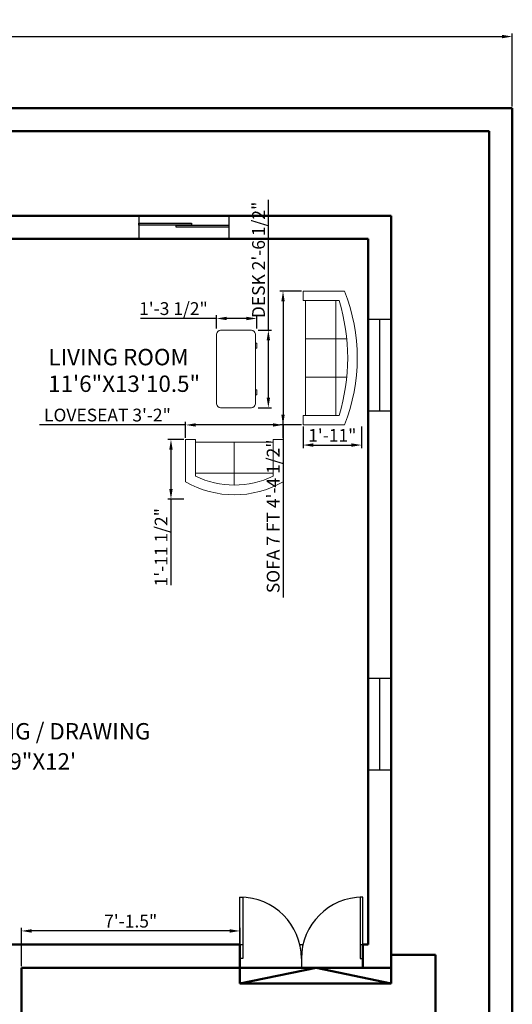
# Model space of a CAD drawing. Units: inches. Extents: x 116541 to 117938, y 135634 to 136328.
# Tile 4 of 9: x 116838 to 117030, y 135936 to 136321. Entities that reach past the tile are written whole.
import ezdxf

# ---------------------------------------------------------------- set-up
doc = ezdxf.new("R2010")
doc.units = ezdxf.units.IN
for name, color, linetype, lineweight in [('A-ANNO-DIMS', 2, 'Continuous', 18), ('A-AREA-IDEN', 3, 'Continuous', 25), ('A-DOOR', 4, 'Continuous', 25), ('A-FURN', 8, 'Continuous', 18), ('A-GLAZ', 1, 'Continuous', 25), ('A-WALL', 7, 'Continuous', 50)]:
    doc.layers.add(name, color=color, linetype=linetype, lineweight=lineweight)
doc.styles.get("Standard").update_dxf_attribs({"font": 'arial.ttf'})
doc.dimstyles.new('ISO-25', dxfattribs={"dimtxt": 5, "dimasz": 4, "dimexe": 1.25, "dimexo": 0.625, "dimtad": 1, "dimdec": 3, "dimlunit": 3, "dimtxsty": 'Standard', "dimcen": 2.5, "dimadec": 0, "dimazin": 0, "dimtfac": 1, "dimtdec": 3, "dimtmove": 0, "dimatfit": 3, "dimfxl": 1, "dimarcsym": 0})

# ---------------------------------------------------------------- blocks, each defined once
blk = doc.blocks.new('*U2')
for p, q in [((0, 0), (0, -6)), ((40, 0), (40, -6))]:
    blk.add_line(p, q)
blk.add_lwpolyline([(0, 0), (0, 40), (1.75, 40), (1.75, 0)], close=True)
blk.add_arc((0, 0), 40, 0, 90)
blk = doc.blocks.new('*U3')
for p, q in [((0, 0), (0, -6)), ((-40, 0), (-40, -6))]:
    blk.add_line(p, q)
blk.add_lwpolyline([(0, 0), (0, 40), (-1.75, 40), (-1.75, 0)], close=True)
blk.add_arc((0, 0), 40, 90, 180)
blk = doc.blocks.new('Sofa - Roundback 7 ft.')
for p, q in [((-36.000027, -34), (-36.000027, -11.4696)), ((-12.00002, -32.4421), (-12.00003, -6.5971)), ((11.99997, -32.4421), (11.99998, -6.5971)), ((35.99998, -34), (35.99998, -11.4696)), ((-35.999844, -13.3819), (35.9998, -13.3819)), ((-36.000027, -32.4421), (35.99998, -32.4421))]:
    blk.add_line(p, q)
for points in [[(-36.000027, -34), (-42.000027, -34), (-42.000027, -8)], [(41.99998, -8), (41.99998, -34), (35.99998, -34)]]:
    blk.add_lwpolyline(points)
for centre, radius, start, end in [((0, -114.25), 114.25, 68.43141, 111.5686), ((-0.00001, -127.1968), 121.1968, 72.72033, 107.2797)]:
    blk.add_arc(centre, radius, start, end)
blk = doc.blocks.new('Sofa - Roundback Loveseat 5 ft.')
for p, q in [((0, -32.44198), (0, -5.99998)), ((-24, -33.99998), (-24, -11.46958)), ((24.00004, -33.99998), (24.00004, -11.46958)), ((-23.9998, -13.38178), (23.99986, -13.38178)), ((-24, -32.44198), (24.00004, -32.44198))]:
    blk.add_line(p, q)
for points in [[(-24, -33.99998), (-30, -33.99998), (-30, -7.99998)], [(30.00004, -7.99998), (30.00004, -33.99998), (24.00004, -33.99998)]]:
    blk.add_lwpolyline(points)
for centre, radius, start, end in [((0, -60.24998), 60.24998, 60.13715, 119.8628), ((0, -61.38438), 55.38444, 64.32083, 115.6792)]:
    blk.add_arc(centre, radius, start, end)
blk = doc.blocks.new('Desk - 30 x 60 in.')
for p, q in [((-26.999995, 0), (26.999995, 0)), ((-29.999995, -27), (-29.999995, -3)), ((29.999995, -3), (29.999995, -27)), ((26.999995, -30), (-26.999995, -30)), ((-20.000005, -30), (-20.000005, -31)), ((-16.000005, -31), (-16.000005, -30)), ((15.999995, -31), (15.999995, -30)), ((19.999995, -30), (19.999995, -31)), ((-20.000005, -31), (-16.000005, -31)), ((19.999995, -31), (15.999995, -31))]:
    blk.add_line(p, q)
for centre, start, end in [((-26.499995, -3.5), 98.1301, 171.8699), ((26.499995, -3.5), 8.130102, 81.8699), ((-26.499995, -26.5), 188.1301, 261.8699), ((26.499995, -26.5), 278.1301, 351.8699)]:
    blk.add_arc(centre, 3.535534, start, end)
blk = doc.blocks.new('*D27')
at = {"layer": 'A-ANNO-DIMS', "color": 0, "lineweight": -2, "transparency": 16777216}
for p, q in [((116583.18, 136287.13), (116583.18, 136315.79)), ((116587.18, 136314.54), (117026.18, 136314.54)), ((117030.18, 136287.13), (117030.18, 136315.79))]:
    blk.add_line(p, q, dxfattribs=at)
at = {"layer": 'A-ANNO-DIMS', "color": 0, "transparency": 16777216}
for points in [[(116587.18, 136315.21), (116587.18, 136313.88), (116583.18, 136314.54)], [(117026.18, 136315.21), (117026.18, 136313.88), (117030.18, 136314.54)]]:
    blk.add_solid(points, dxfattribs=at)
at = {"layer": 'Defpoints', "color": 0, "transparency": 16777216}
for p in [(117030.18, 136314.54), (116583.18, 136286.5), (117030.18, 136286.5)]:
    blk.add_point(p, dxfattribs=at)
at = {"layer": 'A-ANNO-DIMS', "color": 0, "transparency": 16777216, "insert": (116806.68, 136317.72), "char_height": 5, "attachment_point": 5}
blk.add_mtext('37\'-3"', dxfattribs=at)
blk = doc.blocks.new('*D28')
at = {"layer": 'A-ANNO-DIMS', "color": 0, "lineweight": -2, "transparency": 16777216}
for p, q in [((116838.18, 135951.13), (116838.18, 135966.12)), ((116923.68, 135951.13), (116923.68, 135966.12)), ((116919.68, 135964.87), (116842.18, 135964.87))]:
    blk.add_line(p, q, dxfattribs=at)
at = {"layer": 'A-ANNO-DIMS', "color": 0, "transparency": 16777216}
for points in [[(116842.18, 135965.54), (116842.18, 135964.2), (116838.18, 135964.87)], [(116919.68, 135965.54), (116919.68, 135964.2), (116923.68, 135964.87)]]:
    blk.add_solid(points, dxfattribs=at)
at = {"layer": 'Defpoints', "color": 0, "transparency": 16777216}
for p in [(116838.18, 135964.87), (116838.18, 135950.5), (116923.68, 135950.5)]:
    blk.add_point(p, dxfattribs=at)
at = {"layer": 'A-ANNO-DIMS', "color": 0, "transparency": 16777216, "insert": (116880.93, 135968.05), "char_height": 5, "attachment_point": 5}
blk.add_mtext('7\'-1.5"', dxfattribs=at)
blk = doc.blocks.new('*D88')
at = {"layer": 'A-ANNO-DIMS', "color": 0, "lineweight": -2, "transparency": 16777216}
for p, q in [((116947.73, 136215.04), (116939.25, 136215.04)), ((116940.5, 136211.04), (116940.5, 136166.68)), ((116947.73, 136162.68), (116939.25, 136162.68)), ((116940.5, 136162.68), (116940.5, 136095.26))]:
    blk.add_line(p, q, dxfattribs=at)
at = {"layer": 'A-ANNO-DIMS', "color": 0, "transparency": 16777216}
for points in [[(116939.84, 136211.04), (116941.17, 136211.04), (116940.5, 136215.04)], [(116939.84, 136166.68), (116941.17, 136166.68), (116940.5, 136162.68)]]:
    blk.add_solid(points, dxfattribs=at)
at = {"layer": 'Defpoints', "color": 0, "transparency": 16777216}
for p in [(116948.36, 136215.04), (116940.5, 136162.68), (116948.36, 136162.68)]:
    blk.add_point(p, dxfattribs=at)
at = {"layer": 'A-ANNO-DIMS', "color": 0, "transparency": 16777216, "insert": (116937.29, 136126.97), "char_height": 5, "attachment_point": 5, "rotation": 90}
blk.add_mtext('SOFA 7 FT 4\'-4 1/2"', dxfattribs=at)
blk = doc.blocks.new('*D89')
at = {"layer": 'A-ANNO-DIMS', "color": 0, "lineweight": -2, "transparency": 16777216}
for p, q in [((116948.36, 136162.06), (116948.36, 136153.58)), ((116971.21, 136162.06), (116971.21, 136153.58)), ((116952.36, 136154.83), (116967.21, 136154.83))]:
    blk.add_line(p, q, dxfattribs=at)
at = {"layer": 'A-ANNO-DIMS', "color": 0, "transparency": 16777216}
for points in [[(116952.36, 136155.5), (116952.36, 136154.16), (116948.36, 136154.83)], [(116967.21, 136155.5), (116967.21, 136154.16), (116971.21, 136154.83)]]:
    blk.add_solid(points, dxfattribs=at)
at = {"layer": 'Defpoints', "color": 0, "transparency": 16777216}
for p in [(116948.36, 136162.68), (116971.21, 136162.68), (116971.21, 136154.83)]:
    blk.add_point(p, dxfattribs=at)
at = {"layer": 'A-ANNO-DIMS', "color": 0, "transparency": 16777216, "insert": (116959.78, 136157.97), "char_height": 5, "attachment_point": 5}
blk.add_mtext('1\'-11"', dxfattribs=at)
blk = doc.blocks.new('*D90')
at = {"layer": 'A-ANNO-DIMS', "color": 0, "lineweight": -2, "transparency": 16777216}
for p, q in [((116902.4, 136162.69), (116845.26, 136162.69)), ((116902.4, 136157.6), (116902.4, 136163.94)), ((116936.52, 136162.69), (116906.4, 136162.69)), ((116940.52, 136157.6), (116940.52, 136163.94))]:
    blk.add_line(p, q, dxfattribs=at)
at = {"layer": 'A-ANNO-DIMS', "color": 0, "transparency": 16777216}
for points in [[(116906.4, 136163.36), (116906.4, 136162.03), (116902.4, 136162.69)], [(116936.52, 136163.36), (116936.52, 136162.03), (116940.52, 136162.69)]]:
    blk.add_solid(points, dxfattribs=at)
at = {"layer": 'Defpoints', "color": 0, "transparency": 16777216}
for p in [(116902.4, 136162.69), (116902.4, 136156.97), (116940.52, 136156.97)]:
    blk.add_point(p, dxfattribs=at)
at = {"layer": 'A-ANNO-DIMS', "color": 0, "transparency": 16777216, "insert": (116871.83, 136165.91), "char_height": 5, "attachment_point": 5}
blk.add_mtext('LOVESEAT 3\'-2"', dxfattribs=at)
blk = doc.blocks.new('*D91')
at = {"layer": 'A-ANNO-DIMS', "color": 0, "lineweight": -2, "transparency": 16777216}
for p, q in [((116901.77, 136156.97), (116895.43, 136156.97)), ((116896.68, 136152.97), (116896.68, 136137.68)), ((116901.77, 136133.68), (116895.43, 136133.68)), ((116896.68, 136133.68), (116896.68, 136100.07))]:
    blk.add_line(p, q, dxfattribs=at)
at = {"layer": 'A-ANNO-DIMS', "color": 0, "transparency": 16777216}
for points in [[(116896.01, 136152.97), (116897.35, 136152.97), (116896.68, 136156.97)], [(116896.01, 136137.68), (116897.35, 136137.68), (116896.68, 136133.68)]]:
    blk.add_solid(points, dxfattribs=at)
at = {"layer": 'Defpoints', "color": 0, "transparency": 16777216}
for p in [(116902.4, 136156.97), (116896.68, 136133.68), (116902.4, 136133.68)]:
    blk.add_point(p, dxfattribs=at)
at = {"layer": 'A-ANNO-DIMS', "color": 0, "transparency": 16777216, "insert": (116893.47, 136114.88), "char_height": 5, "attachment_point": 5, "rotation": 90}
blk.add_mtext('1\'-11 1/2"', dxfattribs=at)
blk = doc.blocks.new('*D92')
at = {"layer": 'A-ANNO-DIMS', "color": 0, "lineweight": -2, "transparency": 16777216}
for p, q in [((116934.77, 136199.76), (116934.77, 136250.66)), ((116930.84, 136199.76), (116936.02, 136199.76)), ((116934.77, 136173.37), (116934.77, 136195.76)), ((116930.84, 136169.37), (116936.02, 136169.37))]:
    blk.add_line(p, q, dxfattribs=at)
at = {"layer": 'A-ANNO-DIMS', "color": 0, "transparency": 16777216}
for points in [[(116934.1, 136195.76), (116935.44, 136195.76), (116934.77, 136199.76)], [(116934.1, 136173.37), (116935.44, 136173.37), (116934.77, 136169.37)]]:
    blk.add_solid(points, dxfattribs=at)
at = {"layer": 'Defpoints', "color": 0, "transparency": 16777216}
for p in [(116930.21, 136199.76), (116934.77, 136199.76), (116930.21, 136169.37)]:
    blk.add_point(p, dxfattribs=at)
at = {"layer": 'A-ANNO-DIMS', "color": 0, "transparency": 16777216, "insert": (116931.56, 136227.21), "char_height": 5, "attachment_point": 5, "rotation": 90}
blk.add_mtext('DESK 2\'-6 1/2"', dxfattribs=at)
blk = doc.blocks.new('*D93')
at = {"layer": 'A-ANNO-DIMS', "color": 0, "lineweight": -2, "transparency": 16777216}
for p, q in [((116914.51, 136200.38), (116914.51, 136205.57)), ((116930.21, 136200.38), (116930.21, 136205.57)), ((116914.51, 136204.32), (116884.79, 136204.32)), ((116926.21, 136204.32), (116918.51, 136204.32))]:
    blk.add_line(p, q, dxfattribs=at)
at = {"layer": 'A-ANNO-DIMS', "color": 0, "transparency": 16777216}
for points in [[(116918.51, 136204.98), (116918.51, 136203.65), (116914.51, 136204.32)], [(116926.21, 136204.98), (116926.21, 136203.65), (116930.21, 136204.32)]]:
    blk.add_solid(points, dxfattribs=at)
at = {"layer": 'Defpoints', "color": 0, "transparency": 16777216}
for p in [(116914.51, 136204.32), (116914.51, 136199.76), (116930.21, 136199.76)]:
    blk.add_point(p, dxfattribs=at)
at = {"layer": 'A-ANNO-DIMS', "color": 0, "transparency": 16777216, "insert": (116897.65, 136207.53), "char_height": 5, "attachment_point": 5}
blk.add_mtext('1\'-3 1/2"', dxfattribs=at)

msp = doc.modelspace()

# ---------------------------------------------------------------- linework, layer by layer
at = {"layer": 'A-DOOR'}
for points in [[(116923.6763, 135950.5034), (116923.6763, 135959.5034), (116924.7263, 135959.5034)], [(116947.0609, 135959.5034), (116948.2917, 135959.5034)], [(116970.6263, 135959.5034), (116971.6763, 135959.5034), (116971.6763, 135950.5034)]]:
    msp.add_lwpolyline(points, dxfattribs=at)
at = {"layer": 'A-GLAZ'}
for p, q in [((116884.1499, 136244.5034), (116884.1499, 136235.5034)), ((116919.2858, 136244.5436), (116919.2858, 136235.5436)), ((116978.2496, 136204.0672), (116978.2496, 136168.0672)), ((116978.2496, 136063.6641), (116978.2496, 136027.6641))]:
    msp.add_line(p, q, dxfattribs=at)
for points in [[(116884.1499, 136241.6402), (116904.7439, 136241.6402), (116904.7439, 136240.835), (116884.1499, 136240.835)], [(116898.6918, 136240.8488), (116919.2858, 136240.8488), (116919.2858, 136240.0436), (116898.6918, 136240.0436)], [(116973.7496, 136204.0672), (116982.7496, 136204.0672), (116982.7496, 136168.0672), (116973.7496, 136168.0672)], [(116973.7496, 136063.6641), (116982.7496, 136063.6641), (116982.7496, 136027.6641), (116973.7496, 136027.6641)]]:
    msp.add_lwpolyline(points, close=True, dxfattribs=at)
at = {"layer": 'A-WALL'}
for p, q in [((116583.1763, 136286.5034), (117000.1763, 136286.5034)), ((117000.1763, 136286.5034), (117030.1763, 136286.5034)), ((117030.1763, 136286.5034), (117030.1763, 135734.5034)), ((117030.1763, 136286.5034), (117030.1763, 136244.5034)), ((116592.1763, 136277.5034), (117000.1763, 136277.5034)), ((117000.1763, 136277.5034), (117021.1763, 136277.5034)), ((117021.1763, 136277.5034), (117021.1763, 136244.5034)), ((116625.1763, 136244.5034), (116982.7496, 136244.5034)), ((116982.7496, 135944.3286), (116982.7496, 136244.5034)), ((117021.1763, 136244.5034), (117021.1763, 135750.0323)), ((116830.1763, 136235.5034), (116973.7496, 136235.5034)), ((116973.7496, 135959.5034), (116973.7496, 136235.5034)), ((116773.1763, 135959.5034), (116923.6763, 135959.5034)), ((116923.6763, 135959.5034), (116923.6763, 135950.5034)), ((116971.6763, 135959.5034), (116971.6763, 135950.5034)), ((116971.6763, 135959.5034), (116973.7496, 135959.5034)), ((116982.7496, 135955.5034), (117000.1763, 135955.5034)), ((117000.1763, 135955.5034), (117000.1763, 135783.5034)), ((116838.1763, 135950.5034), (116838.1763, 135783.5034)), ((116838.1763, 135950.5034), (116923.6763, 135950.5034)), ((116923.6763, 135950.5034), (116923.6763, 135944.3286)), ((116923.6763, 135944.3286), (116953.4056, 135950.5034)), ((116923.6763, 135950.5034), (116982.7496, 135950.5034)), ((116947.6763, 135950.5034), (116953.4056, 135950.5034)), ((116953.4056, 135950.5034), (116982.7496, 135944.3286)), ((116982.7496, 135944.3286), (116923.6763, 135944.3286))]:
    msp.add_line(p, q, dxfattribs=at)

# ---------------------------------------------------------------- block references
at = {"layer": 'A-DOOR'}
for name, p, xscale, yscale, zscale in [('*U2', (116923.6763, 135954.1034), 0.5999999999997817, 0.5999999999997817, 0.5999999999997817), ('*U3', (116971.6763, 135954.1034), 0.6, 0.6, 0.6)]:
    msp.add_blockref(name, p, dxfattribs=dict(at, xscale=xscale, yscale=yscale, zscale=zscale))
at = {"layer": 'A-FURN'}
for name, p, xscale, yscale, zscale, rotation in [('Sofa - Roundback 7 ft.', (116969.5493, 136188.8618), 0.6232888707088249, 0.6232888707088249, 0.6232888707088249, 270), ('Desk - 30 x 60 in.', (116914.511, 136184.5612), 0.5065123552388274, 0.5065123552388274, 0.5065123552388274, 90), ('Sofa - Roundback Loveseat 5 ft.', (116921.4598, 136135.3724), 0.6353395764405321, 0.6353395764405321, 0.6353395764405321, 180)]:
    msp.add_blockref(name, p, dxfattribs=dict(at, xscale=xscale, yscale=yscale, zscale=zscale, rotation=rotation))

# ---------------------------------------------------------------- texts
at = {"layer": 'A-AREA-IDEN'}
for s, p in [('LIVING ROOM', (116848.76, 136186.013)), ('11\'6"X13\'10.5"', (116848.6568, 136175.6062)), ('DINNING / DRAWING', (116805.675, 136039.7235)), ('        21\'9"X12\'', (116805.675, 136027.9633))]:
    msp.add_text(s, height=6.408368, dxfattribs=at).set_placement(p)

# ---------------------------------------------------------------- dimensions: what is measured, and where the dimension line sits
at = {"layer": 'A-ANNO-DIMS'}
for base, p1, p2, override, picture, middle in [((117030.1763, 136314.5423), (116583.1763, 136286.5034), (117030.1763, 136286.5034), {"dimclrd": 0, "dimclre": 0, "dimclrt": 0}, '*D27', (116806.6763, 136317.7219)), ((116971.2114, 136154.8303), (116948.3575, 136162.6837), (116971.2114, 136162.6837), {"dimdec": 1, "dimrnd": 0, "dimzin": 1, "dimlunit": 4, "dimfrac": 2}, '*D89', (116959.7845, 136157.9655)), ((116838.1763, 135964.8716), (116923.6763, 135950.5034), (116838.1763, 135950.5034), {"dimclrd": 0, "dimclre": 0, "dimclrt": 0}, '*D28', (116880.9263, 135968.0495))]:
    dim = msp.add_linear_dim(base=base, p1=p1, p2=p2, dimstyle='ISO-25', override=override, dxfattribs=at)
    dim.commit()
    dim.dimension.update_dxf_attribs({"geometry": picture, "text_midpoint": middle})
for base, p1, p2, angle, text, picture, middle in [((116934.7715, 136199.7565), (116930.2129, 136169.3658), (116930.2129, 136199.7565), 90, 'DESK <>', '*D92', (116931.5612, 136227.209)), ((116940.5041, 136162.6837), (116948.3575, 136215.04), (116948.3575, 136162.6837), 270, 'SOFA 7 FT <>', '*D88', (116937.2921, 136126.9707)), ((116902.3996, 136162.692), (116940.52, 136156.974), (116902.3996, 136156.974), 180, 'LOVESEAT <>', '*D90', (116871.8298, 136165.9057))]:
    dim = msp.add_linear_dim(base=base, p1=p1, p2=p2, angle=angle, text=text, dimstyle='ISO-25', override={"dimdec": 1, "dimrnd": 0, "dimzin": 1, "dimlunit": 4, "dimfrac": 2}, dxfattribs=at)
    dim.commit()
    dim.dimension.update_dxf_attribs({"geometry": picture, "text_midpoint": middle})
for base, p1, p2, angle, picture, middle in [((116914.511, 136204.3152), (116930.2129, 136199.7565), (116914.511, 136199.7565), 180, '*D93', (116897.6503, 136207.5271)), ((116896.6815, 136133.6782), (116902.3996, 136156.974), (116902.3996, 136133.6782), 270, '*D91', (116893.4712, 136114.8751))]:
    dim = msp.add_linear_dim(base=base, p1=p1, p2=p2, angle=angle, dimstyle='ISO-25', override={"dimdec": 1, "dimrnd": 0, "dimzin": 1, "dimlunit": 4, "dimfrac": 2}, dxfattribs=at)
    dim.commit()
    dim.dimension.update_dxf_attribs({"geometry": picture, "text_midpoint": middle})

doc.saveas('drawing.dxf')
